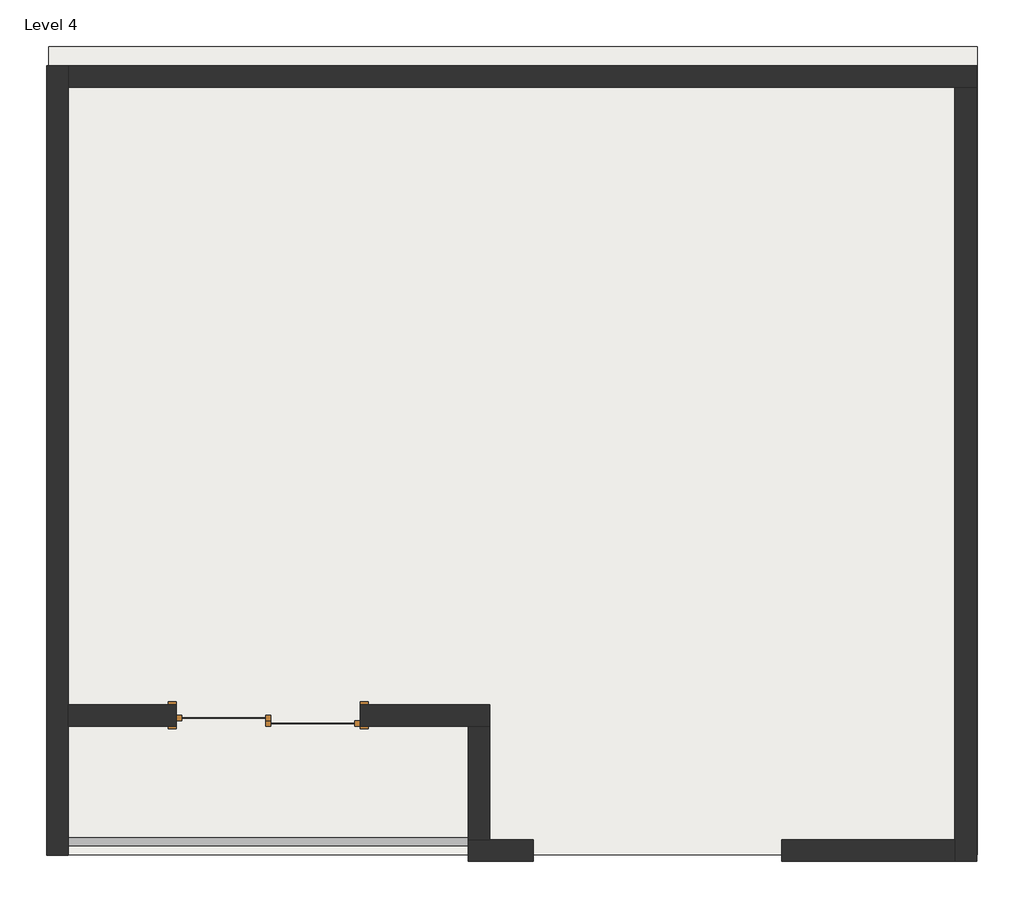
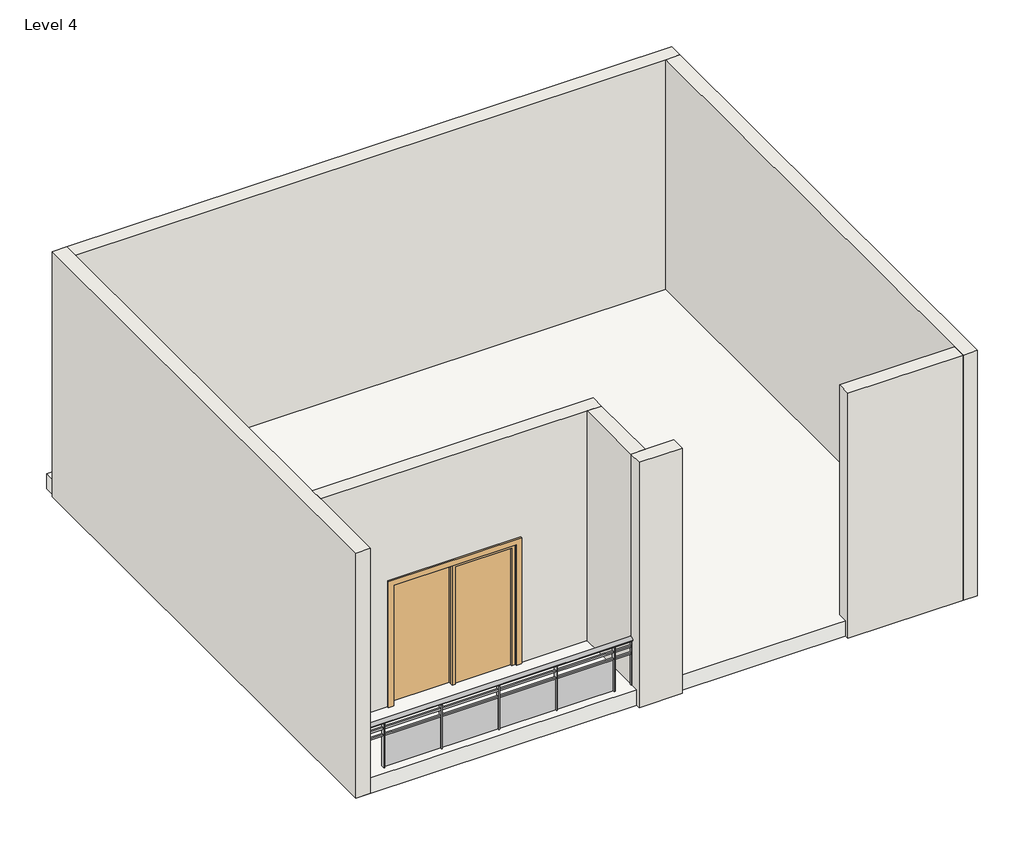
# One storey: 6 walls, 1 door, 1 railing, 1 roof.
"""IFC4 building model written with IfcOpenShell, lengths in millimetres."""

from ifc_helpers import new_model, si_unit, point, frame, origin, place, context, project, spatial, polyline, ellipse_curve, trimmed, outline, extrude, faceted_brep, transform, mapped, element, save
from ifc_brep_helpers import plane_surface, extruded_surface, advanced_brep
from components import door_076b30e0

model = new_model("IFC4")

# Units and contexts
model_context = context("Model", 3, world=origin())
ifc_project = project(units=[si_unit("LENGTHUNIT", "METRE", prefix="MILLI")], contexts=[model_context])

# Site, building, storey
site = spatial("IfcSite", under=ifc_project)
building = spatial("IfcBuilding", under=site)
storey = spatial("IfcBuildingStorey", under=building, Name="Level 4", Elevation=10972.8)

# Door
placement = place(None, origin())
door_shape = door_076b30e0(model_context)
element("IfcDoor", 1, ObjectType="Door-Double-Sliding : 68\" x 80\"", at=placement, inside=storey, context=model_context, shape_type="MappedRepresentation", body=[
    mapped(door_shape, transform((-12373.432922, 6303.7117654, 10972.8), x_axis=(-1.0, 0.0, 0.0), y_axis=(0.0, -1.0, 0.0), z_axis=(0.0, 0.0, 1.0))),
])

# Railing
element("IfcRailing", 2, ObjectType="Glass Panel - Bottom Fill", at=placement, inside=storey, context=model_context, shape_type="SolidModel", body=[
    advanced_brep(
    [(-14253.032922, 5027.3617654, 11887.2), (-14253.032922, 4951.1617654, 11887.2), (-10493.832922, 5027.3617654, 11887.2), (-10493.832922, 4951.1617654, 11887.2)],
    [
        (0, 1, ellipse_curve(frame((-14253.032922, 4989.2617654, 11887.2), z_axis=(-1.0, 0.0, 0.0), x_axis=(0.0, -1.0, 0.0)), 38.1, 28.575)),
        (1, 0, ellipse_curve(frame((-14253.032922, 4989.2617654, 11887.2), z_axis=(-1.0, 0.0, 0.0), x_axis=(0.0, -1.0, 0.0)), 38.1, 28.575)),
        (2, 3, ellipse_curve(frame((-10493.832922, 4989.2617654, 11887.2), z_axis=(1.0, 0.0, 0.0), x_axis=(0.0, -1.0, 0.0)), 38.1, 28.575)),
        (3, 2, ellipse_curve(frame((-10493.832922, 4989.2617654, 11887.2), z_axis=(1.0, 0.0, 0.0), x_axis=(0.0, -1.0, 0.0)), 38.1, 28.575)),
        (0, 2),
        (3, 1),
    ],
    [
        plane_surface(frame((-14253.032922, 4989.2617654, 11887.2), z_axis=(-1.0, 0.0, 0.0), x_axis=(0.0, 1.0, 0.0))),
        plane_surface(frame((-10493.832922, 4989.2617654, 11887.2), z_axis=(1.0, 0.0, 0.0), x_axis=(0.0, 1.0, 0.0))),
        extruded_surface(trimmed(ellipse_curve(frame((-10493.832922, 4989.2617654, 11887.2), z_axis=(-1.0, 0.0, 0.0), x_axis=(0.0, -1.0, 0.0)), 38.1, 28.575), [point((-10493.832922, 5027.3617654, 11887.2))], [point((-10493.832922, 4951.1617654, 11887.2))], True, "CARTESIAN"), (-3759.2000000000007, 0.0, 0.0), 3759.2000000000007),
        extruded_surface(trimmed(ellipse_curve(frame((-10493.832922, 4989.2617654, 11887.2), z_axis=(-1.0, 0.0, 0.0), x_axis=(0.0, -1.0, 0.0)), 38.1, 28.575), [point((-10493.832922, 4951.1617654, 11887.2))], [point((-10493.832922, 5027.3617654, 11887.2))], True, "CARTESIAN"), (-3759.2000000000007, 0.0, 0.0), 3759.2000000000007),
    ],
    [
        (0, [[1, 2]]),
        (1, [[3, 4]]),
        (2, [[-1, 5, -4, 6]]),
        (3, [[-2, -6, -3, -5]]),
    ],
),
    extrude(outline(polyline([(-14253.032922, 4976.5617654), (-14253.032922, 5001.9617654), (-10493.832922, 5001.9617654), (-10493.832922, 4976.5617654), (-14253.032922, 4976.5617654)])), frame((0.0, 0.0, 11772.9), z_axis=(0.0, 0.0, 1.0), x_axis=(1.0, 0.0, 0.0)), (0.0, 0.0, 1.0), 25.4),
    extrude(outline(polyline([(-14253.032922, 4976.5617654), (-14253.032922, 5001.9617654), (-10493.832922, 5001.9617654), (-10493.832922, 4976.5617654), (-14253.032922, 4976.5617654)])), frame((0.0, 0.0, 11671.3), z_axis=(0.0, 0.0, 1.0), x_axis=(1.0, 0.0, 0.0)), (0.0, 0.0, 1.0), 25.4),
    extrude(outline(polyline([(-10754.182922, 4963.8617654), (-10754.182922, 5014.6617654), (-10741.482922, 5014.6617654), (-10741.482922, 4963.8617654), (-10754.182922, 4963.8617654)])), frame((0.0, 0.0, 10972.8), z_axis=(0.0, 0.0, 1.0), x_axis=(1.0, 0.0, 0.0)), (0.0, 0.0, 1.0), 885.6788223),
    extrude(outline(polyline([(-11560.632922, 4995.7969224), (-10747.832922, 4995.7969224), (-10747.832922, 4989.4469224), (-11560.632922, 4989.4469224), (-11560.632922, 4995.7969224)])), frame((0.0, 0.0, 11074.4), z_axis=(0.0, 0.0, 1.0), x_axis=(1.0, 0.0, 0.0)), (0.0, 0.0, 1.0), 596.9),
    extrude(outline(polyline([(-11566.982922, 4963.8617654), (-11566.982922, 5014.6617654), (-11554.282922, 5014.6617654), (-11554.282922, 4963.8617654), (-11566.982922, 4963.8617654)])), frame((0.0, 0.0, 10972.8), z_axis=(0.0, 0.0, 1.0), x_axis=(1.0, 0.0, 0.0)), (0.0, 0.0, 1.0), 885.6788223),
    extrude(outline(polyline([(-12373.432922, 4995.7969224), (-11560.632922, 4995.7969224), (-11560.632922, 4989.4469224), (-12373.432922, 4989.4469224), (-12373.432922, 4995.7969224)])), frame((0.0, 0.0, 11074.4), z_axis=(0.0, 0.0, 1.0), x_axis=(1.0, 0.0, 0.0)), (0.0, 0.0, 1.0), 596.9),
    extrude(outline(polyline([(-12379.782922, 4963.8617654), (-12379.782922, 5014.6617654), (-12367.082922, 5014.6617654), (-12367.082922, 4963.8617654), (-12379.782922, 4963.8617654)])), frame((0.0, 0.0, 10972.8), z_axis=(0.0, 0.0, 1.0), x_axis=(1.0, 0.0, 0.0)), (0.0, 0.0, 1.0), 885.6788223),
    extrude(outline(polyline([(-13186.232922, 4995.7969224), (-12373.432922, 4995.7969224), (-12373.432922, 4989.4469224), (-13186.232922, 4989.4469224), (-13186.232922, 4995.7969224)])), frame((0.0, 0.0, 11074.4), z_axis=(0.0, 0.0, 1.0), x_axis=(1.0, 0.0, 0.0)), (0.0, 0.0, 1.0), 596.9),
    extrude(outline(polyline([(-13192.582922, 4963.8617654), (-13192.582922, 5014.6617654), (-13179.882922, 5014.6617654), (-13179.882922, 4963.8617654), (-13192.582922, 4963.8617654)])), frame((0.0, 0.0, 10972.8), z_axis=(0.0, 0.0, 1.0), x_axis=(1.0, 0.0, 0.0)), (0.0, 0.0, 1.0), 885.6788223),
    extrude(outline(polyline([(-13999.032922, 4995.7969224), (-13186.232922, 4995.7969224), (-13186.232922, 4989.4469224), (-13999.032922, 4989.4469224), (-13999.032922, 4995.7969224)])), frame((0.0, 0.0, 11074.4), z_axis=(0.0, 0.0, 1.0), x_axis=(1.0, 0.0, 0.0)), (0.0, 0.0, 1.0), 596.9),
    extrude(outline(polyline([(-14005.382922, 4963.8617654), (-14005.382922, 5014.6617654), (-13992.682922, 5014.6617654), (-13992.682922, 4963.8617654), (-14005.382922, 4963.8617654)])), frame((0.0, 0.0, 10972.8), z_axis=(0.0, 0.0, 1.0), x_axis=(1.0, 0.0, 0.0)), (0.0, 0.0, 1.0), 885.6788223),
    extrude(outline(polyline([(-10506.532922, 4979.7367654), (-10506.532922, 4998.7867654), (-10487.482922, 4998.7867654), (-10487.482922, 4979.7367654), (-10506.532922, 4979.7367654)])), frame((0.0, 0.0, 10972.8), z_axis=(0.0, 0.0, 1.0), x_axis=(1.0, 0.0, 0.0)), (0.0, 0.0, 1.0), 885.6788223),
    extrude(outline(polyline([(-14259.382922, 4979.7367654), (-14259.382922, 4998.7867654), (-14240.332922, 4998.7867654), (-14240.332922, 4979.7367654), (-14259.382922, 4979.7367654)])), frame((0.0, 0.0, 10972.8), z_axis=(0.0, 0.0, 1.0), x_axis=(1.0, 0.0, 0.0)), (0.0, 0.0, 1.0), 885.6788223),
])

# Roof
element("IfcRoof", 3, ObjectType="Generic - 9\"", at=placement, inside=storey, context=model_context, shape_type="SweptSolid", body=[
    extrude(outline(polyline([(-14435.2593035, 12460.3935836), (-5710.3593035, 12460.3935836), (-5710.3593035, 4865.7935836), (-10301.4093035, 4865.7935836), (-14435.2593035, 4865.7935836), (-14435.2593035, 12460.3935836)])), frame((0.0, 0.0, 10972.8), z_axis=(0.0, 0.0, 1.0), x_axis=(1.0, 0.0, 0.0)), (0.0, 0.0, 1.0), 228.6),
])

# Walls
element("IfcWall", 4, ObjectType="Generic - 8\"", at=placement, inside=storey, context=model_context, shape_type="Brep", body=[
    faceted_brep([(-14253.032922, 4862.2617654, 10972.8), (-14253.032922, 6075.1117654, 10972.8), (-14253.032922, 6278.3117654, 10972.8), (-14253.032922, 12075.8617654, 10972.8), (-14253.032922, 12279.0617654, 10972.8), (-14253.032922, 12279.0617654, 14630.4), (-14253.032922, 12075.8617654, 14630.4), (-14253.032922, 6278.3117654, 14630.4), (-14253.032922, 6075.1117654, 14630.4), (-14253.032922, 4862.2617654, 14630.4), (-14456.232922, 4862.2617654, 10972.8), (-14456.232922, 4862.2617654, 13372.8896509), (-14456.232922, 4862.2617654, 14630.4), (-14456.232922, 12279.0617654, 14630.4), (-14456.232922, 12279.0617654, 10972.8)], [[[0, 1, 2, 3, 4, 5, 6, 7, 8, 9]], [[10, 11, 12, 13, 14]], [[4, 3, 2, 1, 0, 10, 14]], [[9, 8, 7, 6, 5, 13, 12]], [[0, 9, 12, 11, 10]], [[4, 14, 13, 5]]]),
])
element("IfcWall", 5, ObjectType="Generic - 8\"", at=placement, inside=storey, context=model_context, shape_type="Brep", body=[
    faceted_brep([(-14253.032922, 12075.8617654, 14630.4), (-14253.032922, 12075.8617654, 10972.8), (-5921.832922, 12075.8617654, 10972.8), (-5718.632922, 12075.8617654, 10972.8), (-5718.632922, 12075.8617654, 14630.4), (-5921.832922, 12075.8617654, 14630.4), (-14253.032922, 12279.0617654, 10972.8), (-14253.032922, 12279.0617654, 14630.4), (-5718.632922, 12279.0617654, 14630.4), (-5718.632922, 12279.0617654, 10972.8)], [[[0, 1, 2, 3, 4, 5]], [[6, 7, 8, 9]], [[3, 2, 1, 6, 9]], [[0, 5, 4, 8, 7]], [[4, 3, 9, 8]], [[0, 7, 6, 1]]]),
])
element("IfcWall", 6, ObjectType="Generic - 8\"", at=placement, inside=storey, context=model_context, shape_type="Brep", body=[
    faceted_brep([(-5921.832922, 12075.8617654, 10972.8), (-5921.832922, 5008.3117654, 10972.8), (-5921.832922, 4805.1117654, 10972.8), (-5921.832922, 4805.1117654, 14630.4), (-5921.832922, 5008.3117654, 14630.4), (-5921.832922, 12075.8617654, 14630.4), (-5718.632922, 12075.8617654, 10972.8), (-5718.632922, 12075.8617654, 14630.4), (-5718.632922, 4805.1117654, 14630.4), (-5718.632922, 4805.1117654, 10972.8)], [[[0, 1, 2, 3, 4, 5]], [[6, 7, 8, 9]], [[2, 1, 0, 6, 9]], [[5, 4, 3, 8, 7]], [[0, 5, 7, 6]], [[3, 2, 9, 8]]]),
])
element("IfcWall", 7, ObjectType="Generic - 8\"", at=placement, inside=storey, context=model_context, shape_type="Brep", body=[
    faceted_brep([(-5921.832922, 5008.3117654, 10972.8), (-7547.432922, 5008.3117654, 10972.8), (-7547.432922, 5008.3117654, 14630.4), (-5921.832922, 5008.3117654, 14630.4), (-5921.832922, 4805.1117654, 10972.8), (-5921.832922, 4805.1117654, 14630.4), (-7547.432922, 4805.1117654, 14630.4), (-7547.432922, 4805.1117654, 10972.8)], [[[0, 1, 2, 3]], [[4, 5, 6, 7]], [[0, 3, 5, 4]], [[1, 0, 4, 7]], [[2, 1, 7, 6]], [[3, 2, 6, 5]]]),
    faceted_brep([(-10493.832922, 5008.3117654, 14630.4), (-10290.632922, 5008.3117654, 14630.4), (-9884.232922, 5008.3117654, 14630.4), (-9884.232922, 5008.3117654, 10972.8), (-10290.632922, 5008.3117654, 10972.8), (-10493.832922, 5008.3117654, 10972.8), (-10493.832922, 4805.1117654, 14630.4), (-10493.832922, 4805.1117654, 10972.8), (-9884.232922, 4805.1117654, 10972.8), (-9884.232922, 4805.1117654, 14630.4)], [[[0, 1, 2, 3, 4, 5]], [[6, 7, 8, 9]], [[0, 5, 7, 6]], [[2, 1, 0, 6, 9]], [[3, 2, 9, 8]], [[5, 4, 3, 8, 7]]]),
])
element("IfcWall", 8, ObjectType="Generic - 8\"", at=placement, inside=storey, context=model_context, shape_type="Brep", body=[
    faceted_brep([(-14253.032922, 6075.1117654, 10972.8), (-13237.032922, 6075.1117654, 10972.8), (-13237.032922, 6075.1117654, 13004.8), (-11509.832922, 6075.1117654, 13004.8), (-11509.832922, 6075.1117654, 10972.8), (-10493.832922, 6075.1117654, 10972.8), (-10290.632922, 6075.1117654, 10972.8), (-10290.632922, 6075.1117654, 14630.4), (-10493.832922, 6075.1117654, 14630.4), (-14253.032922, 6075.1117654, 14630.4), (-13237.032922, 6278.3117654, 13004.8), (-13237.032922, 6278.3117654, 10972.8), (-14253.032922, 6278.3117654, 10972.8), (-14253.032922, 6278.3117654, 14630.4), (-10290.632922, 6278.3117654, 14630.4), (-10290.632922, 6278.3117654, 10972.8), (-11509.832922, 6278.3117654, 10972.8), (-11509.832922, 6278.3117654, 13004.8)], [[[0, 1, 2, 3, 4, 5, 6, 7, 8, 9]], [[10, 11, 12, 13, 14, 15, 16, 17]], [[16, 15, 6, 5, 4]], [[12, 11, 1, 0]], [[9, 8, 7, 14, 13]], [[7, 6, 15, 14]], [[0, 9, 13, 12]], [[4, 3, 17, 16]], [[2, 1, 11, 10]], [[3, 2, 10, 17]]]),
])
element("IfcWall", 9, ObjectType="Generic - 8\"", at=placement, inside=storey, context=model_context, shape_type="SweptSolid", body=[
    extrude(outline(polyline([(-10493.832922, 5008.3117654), (-10493.832922, 6075.1117654), (-10290.632922, 6075.1117654), (-10290.632922, 5008.3117654), (-10493.832922, 5008.3117654)])), frame((0.0, 0.0, 10972.8), z_axis=(0.0, 0.0, 1.0), x_axis=(1.0, 0.0, 0.0)), (0.0, 0.0, 1.0), 3657.6),
])

save(model, "model.ifc")

# Revit data of these elements
# Type "Door-Double-Sliding : 68\" x 80\""
#   Type Mark = "8"
#   Construction Type Id = "opn-d45"
#   Assembly Code = "C1020"
#   Analytic Construction = "Wood frame, double glass door "
#   Thickness = 0' - 2"
#   Thermal Resistance (R) = 1.8150 (h·ft²·°F)/BTU
#   Heat Transfer Coefficient (U) = 0.5510 BTU/(h·ft²·°F)
#   Height = 6' - 8"
#   Rail Width = 0' - 2"
#   Stiles = 0' - 2"
#   Trim Projection Ext = 0' - 1"
#   Trim Projection Int = 0' - 1"
#   Trim Width = 0' - 3"
#   Width = 5' - 8"
#   Define Thermal Properties by = 1
#   Glazing = Glass
#   Panel Material = Wood - Birch - Solid Stained Light Low Gloss
#   Trim Material = Paint - Sienna
#   Visual Light Transmittance = 0
#   Solar Heat Gain Coefficient = 0
#   Function = (empty or 0)
#   Wall Closure = (empty or 0)
# Type "Glass Panel - Bottom Fill"
#   Assembly Code = "C2010400"
#   built-in parameter 1008612 = 0.0416667 (stored number, unit not read)
#   built-in parameter 1008611 = 0.0416667 (stored number, unit not read)
#   built-in parameter 1008609 = 0.333333 (stored number, unit not read)
#   built-in parameter 1008604 = 0.166667 (stored number, unit not read)
#   built-in parameter 1008603 = 0.166667 (stored number, unit not read)
#   Railing Height = 3' - 0"
#   built-in parameter 1008630 = 2
#   built-in parameter 1008610 = 2
#   built-in parameter 1008618 = Baluster - Square : 3/4"
# Type "Generic - 9\""
#   Assembly Code = "B1020"
#   Layers, outside or top first: 0' - 9" no material (function 1)
# Type "Generic - 8\""
#   Assembly Code = "B2010"
#   Layers, outside or top first: 0' - 8" no material (function 1)
# Element 1 (IfcDoor, "Door-Double-Sliding : 68\" x 80\"")
#   Phase Created = New Construction
#   Materials on its faces: "Paint - Sienna", "Wood - Birch - Solid Stained Light Low Gloss", "Glass"
# Element 2 (IfcRailing, "Glass Panel - Bottom Fill")
#   Phase Created = New Construction
#   Materials on its faces: "Glass"
# Element 3 (IfcRoof, "Generic - 9\"")
#   built-in parameter 1001705 = 36.75 (stored number, unit not read)
#   built-in parameter 1001710 = 33615
#   Phase Created = New Construction
#   Materials on its faces: "Default Roof"
# Elements 4, 5, 6, 7, 8, 9 (IfcWall, "Generic - 8\"")
#   Top Offset = 0' - 0"
#   Base Offset = 0' - 0"
#   Unconnected Height = 12' - 0"
#   wall height = 12' - 0"
#   Phase Created = New Construction
#   Base Constraint = Level 4
#   Materials on its faces: "Default Wall"
# Materials
#   "Glass": class "Glass", colour RGB 0 128 192, transparency 0.75, Description = "Soda Lime Glass", Cost = 0
#   "Wood - Birch - Solid Stained Light Low Gloss": class "Wood", colour RGB 210 159 95, transparency 0, Cost = 0
#   "Paint - Sienna": colour RGB 118 70 51, transparency 0, Cost = 0
#   "Default Roof": colour RGB 88 101 114, transparency 0
#   "Default Wall": colour RGB 128 128 128, transparency 0
